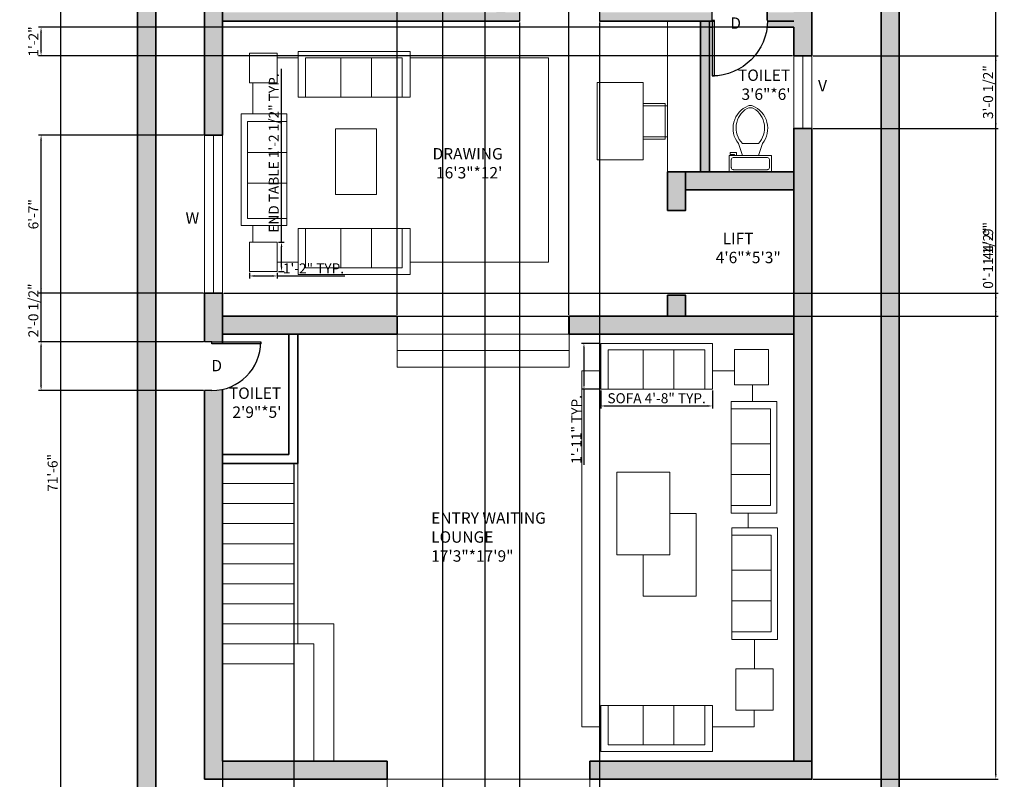
# Model space of a CAD drawing. Units: inches. Extents: x 2130 to 2621, y 981 to 1994.
# Tile 2 of 4: x 2130 to 2621, y 1353 to 1732. Entities that reach past the tile are written whole.
import ezdxf

# ---------------------------------------------------------------- set-up
doc = ezdxf.new("R2010")
doc.units = ezdxf.units.IN
for name, color, linetype, lineweight in [('A-ANNO-DIMS', 2, 'Continuous', 18), ('A-ANNO-TEXT', 10, 'Continuous', 18), ('A-AREA-IDEN', 10, 'Continuous', 18), ('A-FLOR-FIXT', 190, 'Continuous', 18), ('A-FLOR-STRS', 7, 'Continuous', 18), ('A-WALL-PATT', 140, 'Continuous', 13), ('C-PROP', 7, 'Continuous', 35), ('C-PROP-PATT', 140, 'Continuous', 13), ('DOOR', 130, 'Continuous', 25), ('FUR', 190, 'Continuous', 18), ('WALL', 140, 'Continuous', 35), ('WIND', 210, 'Continuous', 18)]:
    doc.layers.add(name, color=color, linetype=linetype, lineweight=lineweight)
doc.styles.get("Standard").update_dxf_attribs({"font": 'arial.ttf'})
doc.dimstyles.new('ISO-25', dxfattribs={"dimtxt": 5, "dimasz": 2.5, "dimexe": 1.25, "dimexo": 0.625, "dimtad": 1, "dimdec": 0, "dimlunit": 4, "dimtxsty": 'Standard', "dimcen": 2.5, "dimadec": 0, "dimazin": 0, "dimtfac": 1, "dimtdec": 0, "dimtmove": 0, "dimatfit": 3, "dimfxl": 1, "dimarcsym": 0})

# ---------------------------------------------------------------- blocks, each defined once
blk = doc.blocks.new('*U2')
for p, q in [((0, 0), (0, -6)), ((40, 0), (40, -6))]:
    blk.add_line(p, q)
blk.add_lwpolyline([(0, 0), (0, 40), (1.75, 40), (1.75, 0)], close=True)
blk.add_arc((0, 0), 40, 0, 90)
blk = doc.blocks.new('*D10')
at = {"layer": 'A-ANNO-DIMS', "color": 0, "lineweight": -2, "transparency": 16777216}
for p, q in [((2188.13, 1935.02), (2148.94, 1935.02)), ((2150.19, 1932.52), (2150.19, 1079.91)), ((2188.13, 1077.41), (2148.94, 1077.41))]:
    blk.add_line(p, q, dxfattribs=at)
at = {"layer": 'A-ANNO-DIMS', "color": 0, "transparency": 16777216}
for points in [[(2149.77, 1932.52), (2150.61, 1932.52), (2150.19, 1935.02)], [(2149.77, 1079.91), (2150.61, 1079.91), (2150.19, 1077.41)]]:
    blk.add_solid(points, dxfattribs=at)
at = {"layer": 'Defpoints', "color": 0, "transparency": 16777216}
for p in [(2188.76, 1935.02), (2150.19, 1077.41), (2188.76, 1077.41)]:
    blk.add_point(p, dxfattribs=at)
at = {"layer": 'A-ANNO-DIMS', "color": 0, "transparency": 16777216, "insert": (2147.01, 1506.21), "char_height": 5, "attachment_point": 5, "rotation": 90}
blk.add_mtext('71\'-6"', dxfattribs=at)
blk = doc.blocks.new('*U4')
for p, q in [((9.5, -6), (9.5, -2)), ((-10, -8.5), (-8, -8.5)), ((-10, -9.5), (-10, -8.5)), ((-7, -9.5), (-10, -9.5)), ((-8, -8.5), (-8, -8)), ((-7, -8), (-7, -9.5)), ((-4, -8), (-6, -14)), ((4, -8), (6, -14)), ((4, -14), (-4, -14))]:
    blk.add_line(p, q)
blk.add_lwpolyline([(10.5, -8), (10.5, 0), (-10.5, 0), (-10.5, -8)], close=True)
for points in [[(-9.5, -2), (-9.5, -6)], [(8.5, -1), (-8.5, -1)], [(-8.5, -7), (8.5, -7)]]:
    blk.add_lwpolyline(points)
for centre, radius, start, end in [((-8.62, -1.88), 0.884, 81.8699, 188.1301), ((8.62, -1.88), 0.884, 351.8699, 98.1301), ((-8.62, -6.12), 0.884, 171.8699, 278.1301), ((8.62, -6.12), 0.884, 261.8699, 8.1301), ((3.52, -21.58), 12.17, 141.4691, 247.9714), ((4.2, -21.82), 11.33, 136.3677, 238.9468), ((-3.52, -21.58), 12.17, 292.0284, 38.5307), ((-4.2, -21.82), 11.33, 301.053, 43.6321), ((0, -27.88), 4, 245.7318, 294.2682), ((0, -29), 4, 254.8605, 285.1395)]:
    blk.add_arc(centre, radius, start, end)
blk = doc.blocks.new('SOFA-THREE-SEAT')
for p, q in [((0, 0), (0, 55.76)), ((0, 55.76), (22.87, 55.76)), ((22.87, 55.76), (22.87, 51.91)), ((3.25, 36.47), (22.87, 36.47)), ((3.25, 21.24), (22.87, 21.24)), ((1.57, 0), (0, 0)), ((22.87, 0), (1.57, 0)), ((22.87, 3.65), (22.87, 0))]:
    blk.add_line(p, q)
blk.add_lwpolyline([(3.25, 3.65), (22.87, 3.65), (22.87, 51.91), (3.25, 51.91)], close=True)
blk = doc.blocks.new('TABLE-END')
blk.add_lwpolyline([(0, 14.67), (13.78, 14.67), (13.78, 0), (0, 0)], close=True)
blk = doc.blocks.new('*D15')
at = {"layer": 'A-ANNO-DIMS', "color": 0, "lineweight": -2, "transparency": 16777216}
for p, q in [((2419.82, 1547.31), (2419.82, 1538.32)), ((2475.58, 1547.31), (2475.58, 1538.32)), ((2422.32, 1539.57), (2473.08, 1539.57))]:
    blk.add_line(p, q, dxfattribs=at)
at = {"layer": 'A-ANNO-DIMS', "color": 0, "transparency": 16777216}
for points in [[(2422.32, 1539.99), (2422.32, 1539.16), (2419.82, 1539.57)], [(2473.08, 1539.99), (2473.08, 1539.16), (2475.58, 1539.57)]]:
    blk.add_solid(points, dxfattribs=at)
at = {"layer": 'Defpoints', "color": 0, "transparency": 16777216}
for p in [(2419.82, 1547.94), (2475.58, 1547.94), (2475.58, 1539.57)]:
    blk.add_point(p, dxfattribs=at)
at = {"layer": 'A-ANNO-DIMS', "color": 0, "transparency": 16777216, "insert": (2447.7, 1542.79), "char_height": 5, "attachment_point": 5}
blk.add_mtext('SOFA 4\'-8" TYP.', dxfattribs=at)
blk = doc.blocks.new('*D16')
at = {"layer": 'A-ANNO-DIMS', "color": 0, "lineweight": -2, "transparency": 16777216}
for p, q in [((2419.19, 1570.81), (2410.2, 1570.81)), ((2411.45, 1568.31), (2411.45, 1550.44)), ((2419.19, 1547.94), (2410.2, 1547.94)), ((2411.45, 1547.94), (2411.45, 1510.3))]:
    blk.add_line(p, q, dxfattribs=at)
at = {"layer": 'A-ANNO-DIMS', "color": 0, "transparency": 16777216}
for points in [[(2411.04, 1568.31), (2411.87, 1568.31), (2411.45, 1570.81)], [(2411.04, 1550.44), (2411.87, 1550.44), (2411.45, 1547.94)]]:
    blk.add_solid(points, dxfattribs=at)
at = {"layer": 'Defpoints', "color": 0, "transparency": 16777216}
for p in [(2419.82, 1570.81), (2411.45, 1547.94), (2419.82, 1547.94)]:
    blk.add_point(p, dxfattribs=at)
at = {"layer": 'A-ANNO-DIMS', "color": 0, "transparency": 16777216, "insert": (2408.32, 1527.87), "char_height": 5, "attachment_point": 5, "rotation": 90}
blk.add_mtext('1\'-11" TYP.', dxfattribs=at)
blk = doc.blocks.new('*D21')
at = {"layer": 'A-ANNO-DIMS', "color": 0, "lineweight": -2, "transparency": 16777216}
for p, q in [((2260.56, 1621.28), (2260.56, 1707.66)), ((2258.99, 1621.28), (2261.81, 1621.28)), ((2260.56, 1609.11), (2260.56, 1618.78)), ((2258.99, 1606.61), (2261.81, 1606.61))]:
    blk.add_line(p, q, dxfattribs=at)
at = {"layer": 'A-ANNO-DIMS', "color": 0, "transparency": 16777216}
for points in [[(2260.15, 1618.78), (2260.98, 1618.78), (2260.56, 1621.28)], [(2260.15, 1609.11), (2260.98, 1609.11), (2260.56, 1606.61)]]:
    blk.add_solid(points, dxfattribs=at)
at = {"layer": 'Defpoints', "color": 0, "transparency": 16777216}
for p in [(2258.36, 1621.28), (2260.56, 1621.28), (2258.36, 1606.61)]:
    blk.add_point(p, dxfattribs=at)
at = {"layer": 'A-ANNO-DIMS', "color": 0, "transparency": 16777216, "insert": (2257.35, 1665.72), "char_height": 5, "attachment_point": 5, "rotation": 90}
blk.add_mtext('END TABLE 1\'-2 1/2" TYP.', dxfattribs=at)
blk = doc.blocks.new('*D22')
at = {"layer": 'A-ANNO-DIMS', "color": 0, "lineweight": -2, "transparency": 16777216}
for p, q in [((2244.58, 1605.98), (2244.58, 1603.16)), ((2247.08, 1604.41), (2255.86, 1604.41)), ((2258.36, 1605.98), (2258.36, 1603.16)), ((2258.36, 1604.41), (2292.12, 1604.41))]:
    blk.add_line(p, q, dxfattribs=at)
at = {"layer": 'A-ANNO-DIMS', "color": 0, "transparency": 16777216}
for points in [[(2247.08, 1604.82), (2247.08, 1603.99), (2244.58, 1604.41)], [(2255.86, 1604.82), (2255.86, 1603.99), (2258.36, 1604.41)]]:
    blk.add_solid(points, dxfattribs=at)
at = {"layer": 'Defpoints', "color": 0, "transparency": 16777216}
for p in [(2244.58, 1606.61), (2258.36, 1606.61), (2258.36, 1604.41)]:
    blk.add_point(p, dxfattribs=at)
at = {"layer": 'A-ANNO-DIMS', "color": 0, "transparency": 16777216, "insert": (2276.49, 1607.54), "char_height": 5, "attachment_point": 5}
blk.add_mtext('1\'-2" TYP.', dxfattribs=at)
blk = doc.blocks.new('*D24')
at = {"layer": 'A-ANNO-DIMS', "color": 0, "lineweight": -2, "transparency": 16777216}
for p, q in [((2525.79, 1890.41), (2618.19, 1890.41)), ((2616.94, 1355.91), (2616.94, 1887.91)), ((2525.79, 1353.41), (2618.19, 1353.41))]:
    blk.add_line(p, q, dxfattribs=at)
at = {"layer": 'A-ANNO-DIMS', "color": 0, "transparency": 16777216}
for points in [[(2616.52, 1887.91), (2617.35, 1887.91), (2616.94, 1890.41)], [(2616.52, 1355.91), (2617.35, 1355.91), (2616.94, 1353.41)]]:
    blk.add_solid(points, dxfattribs=at)
at = {"layer": 'Defpoints', "color": 0, "transparency": 16777216}
for p in [(2525.16, 1890.41), (2616.94, 1890.41), (2525.16, 1353.41)]:
    blk.add_point(p, dxfattribs=at)
at = {"layer": 'A-ANNO-DIMS', "color": 0, "transparency": 16777216, "insert": (2613.76, 1621.91), "char_height": 5, "attachment_point": 5, "rotation": 90}
blk.add_mtext('44\'-9"', dxfattribs=at)
blk = doc.blocks.new('*D32')
at = {"layer": 'A-ANNO-DIMS', "color": 0, "lineweight": -2, "transparency": 16777216}
for p, q in [((2318.23, 1585.04), (2318.23, 1984.45)), ((2320.73, 1983.2), (2401.44, 1983.2)), ((2403.94, 1585.04), (2403.94, 1984.45))]:
    blk.add_line(p, q, dxfattribs=at)
at = {"layer": 'A-ANNO-DIMS', "color": 0, "transparency": 16777216}
for points in [[(2320.73, 1983.61), (2320.73, 1982.78), (2318.23, 1983.2)], [(2401.44, 1983.61), (2401.44, 1982.78), (2403.94, 1983.2)]]:
    blk.add_solid(points, dxfattribs=at)
at = {"layer": 'Defpoints', "color": 0, "transparency": 16777216}
for p in [(2403.94, 1983.2), (2318.23, 1584.41), (2403.94, 1584.41)]:
    blk.add_point(p, dxfattribs=at)
at = {"layer": 'A-ANNO-DIMS', "color": 0, "transparency": 16777216, "insert": (2361.08, 1986.41), "char_height": 5, "attachment_point": 5}
blk.add_mtext('7\'-1 1/2"', dxfattribs=at)
blk = doc.blocks.new('*D33')
at = {"layer": 'A-ANNO-DIMS', "color": 0, "lineweight": -2, "transparency": 16777216}
for p, q in [((2231.16, 1510.29), (2231.16, 984.42)), ((2266.66, 1510.29), (2266.66, 984.42)), ((2233.66, 985.67), (2264.16, 985.67))]:
    blk.add_line(p, q, dxfattribs=at)
at = {"layer": 'A-ANNO-DIMS', "color": 0, "transparency": 16777216}
for points in [[(2233.66, 986.08), (2233.66, 985.25), (2231.16, 985.67)], [(2264.16, 986.08), (2264.16, 985.25), (2266.66, 985.67)]]:
    blk.add_solid(points, dxfattribs=at)
at = {"layer": 'Defpoints', "color": 0, "transparency": 16777216}
for p in [(2231.16, 1510.91), (2266.66, 1510.91), (2266.66, 985.67)]:
    blk.add_point(p, dxfattribs=at)
at = {"layer": 'A-ANNO-DIMS', "color": 0, "transparency": 16777216, "insert": (2248.91, 988.88), "char_height": 5, "attachment_point": 5}
blk.add_mtext('2\'-11 1/2"', dxfattribs=at)
blk = doc.blocks.new('*D36')
at = {"layer": 'A-ANNO-DIMS', "color": 0, "lineweight": -2, "transparency": 16777216}
for p, q in [((2379.27, 1730.79), (2379.27, 984.42)), ((2419.27, 1730.79), (2419.27, 984.42)), ((2381.77, 985.67), (2416.77, 985.67))]:
    blk.add_line(p, q, dxfattribs=at)
at = {"layer": 'A-ANNO-DIMS', "color": 0, "transparency": 16777216}
for points in [[(2381.77, 986.08), (2381.77, 985.25), (2379.27, 985.67)], [(2416.77, 986.08), (2416.77, 985.25), (2419.27, 985.67)]]:
    blk.add_solid(points, dxfattribs=at)
at = {"layer": 'Defpoints', "color": 0, "transparency": 16777216}
for p in [(2379.27, 1731.41), (2419.27, 1731.41), (2419.27, 985.67)]:
    blk.add_point(p, dxfattribs=at)
at = {"layer": 'A-ANNO-DIMS', "color": 0, "transparency": 16777216, "insert": (2399.27, 988.85), "char_height": 5, "attachment_point": 5}
blk.add_mtext('3\'-4"', dxfattribs=at)
blk = doc.blocks.new('*D37')
at = {"layer": 'A-ANNO-DIMS', "color": 0, "lineweight": -2, "transparency": 16777216}
for p, q in [((2475.37, 1732.39), (2475.37, 1984.45)), ((2477.87, 1983.2), (2500.44, 1983.2)), ((2502.94, 1732.04), (2502.94, 1984.45))]:
    blk.add_line(p, q, dxfattribs=at)
at = {"layer": 'A-ANNO-DIMS', "color": 0, "transparency": 16777216}
for points in [[(2477.87, 1983.61), (2477.87, 1982.78), (2475.37, 1983.2)], [(2500.44, 1983.61), (2500.44, 1982.78), (2502.94, 1983.2)]]:
    blk.add_solid(points, dxfattribs=at)
at = {"layer": 'Defpoints', "color": 0, "transparency": 16777216}
for p in [(2502.94, 1983.2), (2475.37, 1731.77), (2502.94, 1731.41)]:
    blk.add_point(p, dxfattribs=at)
at = {"layer": 'A-ANNO-DIMS', "color": 0, "transparency": 16777216, "insert": (2489.15, 1986.41), "char_height": 5, "attachment_point": 5}
blk.add_mtext('2\'-3 1/2"', dxfattribs=at)
blk = doc.blocks.new('*D38')
at = {"layer": 'A-ANNO-DIMS', "color": 0, "lineweight": -2, "transparency": 16777216}
for p, q in [((2140.58, 1571.6), (2140.58, 1600.38)), ((2221.54, 1571.6), (2139.33, 1571.6)), ((2140.58, 1549.77), (2140.58, 1569.1)), ((2221.54, 1547.27), (2139.33, 1547.27))]:
    blk.add_line(p, q, dxfattribs=at)
at = {"layer": 'A-ANNO-DIMS', "color": 0, "transparency": 16777216}
for points in [[(2140.16, 1569.1), (2140.99, 1569.1), (2140.58, 1571.6)], [(2140.16, 1549.77), (2140.99, 1549.77), (2140.58, 1547.27)]]:
    blk.add_solid(points, dxfattribs=at)
at = {"layer": 'Defpoints', "color": 0, "transparency": 16777216}
for p in [(2140.58, 1571.6), (2222.16, 1571.6), (2222.16, 1547.27)]:
    blk.add_point(p, dxfattribs=at)
at = {"layer": 'A-ANNO-DIMS', "color": 0, "transparency": 16777216, "insert": (2137.37, 1587.24), "char_height": 5, "attachment_point": 5, "rotation": 90}
blk.add_mtext('2\'-0 1/2"', dxfattribs=at)
blk = doc.blocks.new('*D42')
at = {"layer": 'A-ANNO-DIMS', "color": 0, "lineweight": -2, "transparency": 16777216}
for p, q in [((2221.54, 1674.58), (2139.33, 1674.58)), ((2140.58, 1598.3), (2140.58, 1672.08)), ((2221.54, 1595.8), (2139.33, 1595.8))]:
    blk.add_line(p, q, dxfattribs=at)
at = {"layer": 'A-ANNO-DIMS', "color": 0, "transparency": 16777216}
for points in [[(2140.16, 1672.08), (2140.99, 1672.08), (2140.58, 1674.58)], [(2140.16, 1598.3), (2140.99, 1598.3), (2140.58, 1595.8)]]:
    blk.add_solid(points, dxfattribs=at)
at = {"layer": 'Defpoints', "color": 0, "transparency": 16777216}
for p in [(2140.58, 1674.58), (2222.16, 1674.58), (2222.16, 1595.8)]:
    blk.add_point(p, dxfattribs=at)
at = {"layer": 'A-ANNO-DIMS', "color": 0, "transparency": 16777216, "insert": (2137.4, 1635.19), "char_height": 5, "attachment_point": 5, "rotation": 90}
blk.add_mtext('6\'-7"', dxfattribs=at)
blk = doc.blocks.new('*D44')
at = {"layer": 'A-ANNO-DIMS', "color": 0, "lineweight": -2, "transparency": 16777216}
for p, q in [((2525.79, 1714.24), (2618.19, 1714.24)), ((2616.94, 1680.45), (2616.94, 1711.74)), ((2525.79, 1677.95), (2618.19, 1677.95))]:
    blk.add_line(p, q, dxfattribs=at)
at = {"layer": 'A-ANNO-DIMS', "color": 0, "transparency": 16777216}
for points in [[(2616.52, 1711.74), (2617.35, 1711.74), (2616.94, 1714.24)], [(2616.52, 1680.45), (2617.35, 1680.45), (2616.94, 1677.95)]]:
    blk.add_solid(points, dxfattribs=at)
at = {"layer": 'Defpoints', "color": 0, "transparency": 16777216}
for p in [(2525.16, 1714.24), (2616.94, 1714.24), (2525.16, 1677.95)]:
    blk.add_point(p, dxfattribs=at)
at = {"layer": 'A-ANNO-DIMS', "color": 0, "transparency": 16777216, "insert": (2613.72, 1696.09), "char_height": 5, "attachment_point": 5, "rotation": 90}
blk.add_mtext('3\'-0 1/2"', dxfattribs=at)
blk = doc.blocks.new('*D45')
at = {"layer": 'A-ANNO-DIMS', "color": 0, "lineweight": -2, "transparency": 16777216}
for p, q in [((2340.91, 1828.29), (2340.91, 984.42)), ((2361.98, 1828.29), (2361.98, 984.42)), ((2343.41, 985.67), (2359.48, 985.67))]:
    blk.add_line(p, q, dxfattribs=at)
at = {"layer": 'A-ANNO-DIMS', "color": 0, "transparency": 16777216}
for points in [[(2343.41, 986.08), (2343.41, 985.25), (2340.91, 985.67)], [(2359.48, 986.08), (2359.48, 985.25), (2361.98, 985.67)]]:
    blk.add_solid(points, dxfattribs=at)
at = {"layer": 'Defpoints', "color": 0, "transparency": 16777216}
for p in [(2340.91, 1828.91), (2361.98, 1828.91), (2361.98, 985.67)]:
    blk.add_point(p, dxfattribs=at)
at = {"layer": 'A-ANNO-DIMS', "color": 0, "transparency": 16777216, "insert": (2351.44, 988.84), "char_height": 5, "attachment_point": 5}
blk.add_mtext('1\'-9"', dxfattribs=at)
blk = doc.blocks.new('*D47')
at = {"layer": 'A-ANNO-DIMS', "color": 0, "lineweight": -2, "transparency": 16777216}
for p, q in [((2616.94, 1595.8), (2616.94, 1628.38)), ((2231.79, 1595.8), (2618.19, 1595.8)), ((2616.94, 1586.91), (2616.94, 1593.3)), ((2231.79, 1584.41), (2618.19, 1584.41))]:
    blk.add_line(p, q, dxfattribs=at)
at = {"layer": 'A-ANNO-DIMS', "color": 0, "transparency": 16777216}
for points in [[(2616.52, 1593.3), (2617.35, 1593.3), (2616.94, 1595.8)], [(2616.52, 1586.91), (2617.35, 1586.91), (2616.94, 1584.41)]]:
    blk.add_solid(points, dxfattribs=at)
at = {"layer": 'Defpoints', "color": 0, "transparency": 16777216}
for p in [(2231.16, 1595.8), (2616.94, 1595.8), (2231.16, 1584.41)]:
    blk.add_point(p, dxfattribs=at)
at = {"layer": 'A-ANNO-DIMS', "color": 0, "transparency": 16777216, "insert": (2613.73, 1613.34), "char_height": 5, "attachment_point": 5, "rotation": 90}
blk.add_mtext('0\'-11 1/2"', dxfattribs=at)
blk = doc.blocks.new('*D54')
at = {"layer": 'A-ANNO-DIMS', "color": 0, "lineweight": -2, "transparency": 16777216}
for p, q in [((2515.54, 1728.41), (2139.33, 1728.41)), ((2140.58, 1716.74), (2140.58, 1725.91)), ((2515.54, 1714.24), (2139.33, 1714.24))]:
    blk.add_line(p, q, dxfattribs=at)
at = {"layer": 'A-ANNO-DIMS', "color": 0, "transparency": 16777216}
for points in [[(2140.16, 1725.91), (2140.99, 1725.91), (2140.58, 1728.41)], [(2140.16, 1716.74), (2140.99, 1716.74), (2140.58, 1714.24)]]:
    blk.add_solid(points, dxfattribs=at)
at = {"layer": 'Defpoints', "color": 0, "transparency": 16777216}
for p in [(2140.58, 1728.41), (2516.16, 1728.41), (2516.16, 1714.24)]:
    blk.add_point(p, dxfattribs=at)
at = {"layer": 'A-ANNO-DIMS', "color": 0, "transparency": 16777216, "insert": (2137.44, 1721.33), "char_height": 5, "attachment_point": 5, "rotation": 90}
blk.add_mtext('1\'-2"', dxfattribs=at)

msp = doc.modelspace()

# ---------------------------------------------------------------- hatches: boundary and pattern name
at = {"layer": 'A-WALL-PATT'}
h = msp.add_hatch(color=256, dxfattribs=at)
h.dxf.hatch_style = 1
h.paths.add_polyline_path([(2272.17, 1886.91), (2272.17, 1890.41), (2222.16, 1890.41), (2222.16, 1870.49), (2231.16, 1870.49), (2231.16, 1881.41), (2272.82, 1881.41, -0.059514)])
h.paths.add_polyline_path([(2231.16, 1828.91), (2301.66, 1828.91), (2301.66, 1881.41), (2297.16, 1881.41), (2297.16, 1833.41), (2265.07, 1833.41), (2231.16, 1833.41), (2231.16, 1841.86), (2222.16, 1841.86), (2222.16, 1828.91), (2222.16, 1790.61), (2228.16, 1790.61, -0.01877), (2231.16, 1790.5)])
h.paths.add_polyline_path([(2303.95, 1886.91), (2303.95, 1890.41), (2301.66, 1890.41), (2295.51, 1890.41), (2295.51, 1886.91), (2295.51, 1881.41), (2297.16, 1881.41), (2301.66, 1881.41), (2303.95, 1881.41)])
h.paths.add_polyline_path([(2525.16, 1890.41), (2372.16, 1890.41), (2327.29, 1890.41), (2327.29, 1886.91, -0.059514), (2326.63, 1881.41), (2367.66, 1881.41), (2367.66, 1833.41), (2361.98, 1833.41), (2361.98, 1828.91), (2367.66, 1828.91), (2367.66, 1735.91), (2372.16, 1735.91), (2372.16, 1828.91), (2372.16, 1881.41), (2516.16, 1881.41), (2516.16, 1859.91), (2516.16, 1809.41), (2525.16, 1809.41)])
h.paths.add_polyline_path([(2475.37, 1735.91), (2419.27, 1735.91), (2419.27, 1731.41), (2475.37, 1731.41), (2475.37, 1731.77)])
h.paths.add_polyline_path([(2525.16, 1751.59), (2516.16, 1751.59), (2516.16, 1737.41), (2516.16, 1735.91), (2503, 1735.91), (2503, 1731.77, -0.030428), (2502.8, 1728.41), (2516.16, 1728.41), (2516.16, 1714.24), (2525.16, 1714.24), (2525.16, 1728.41)])
h.paths.add_polyline_path([(2379.27, 1735.91), (2231.16, 1735.91), (2231.16, 1731.41), (2379.27, 1731.41)])
h.paths.add_polyline_path([(2231.16, 1728.41), (2231.16, 1735.91), (2231.16, 1750.61), (2228.16, 1750.61), (2222.16, 1750.61), (2222.16, 1728.41), (2222.16, 1674.58), (2231.16, 1674.58)])
h.paths.add_polyline_path([(2516.16, 1584.41), (2462.16, 1584.41), (2403.94, 1584.41), (2403.94, 1575.41), (2404.07, 1575.41), (2453.16, 1575.41), (2516.16, 1575.41)], flags=17)
h.paths.add_polyline_path([(2516.16, 1584.41), (2462.16, 1584.41), (2403.94, 1584.41), (2403.94, 1575.41), (2453.16, 1575.41), (2516.16, 1575.41)], flags=17)
h.paths.add_polyline_path([(2318.23, 1584.41), (2231.16, 1584.41), (2231.16, 1575.41), (2318.23, 1575.41)])
h = msp.add_hatch(color=256, dxfattribs=at)
h.dxf.hatch_style = 1
h.paths.add_polyline_path([(2231.16, 1595.8), (2222.16, 1595.8), (2222.16, 1571.6), (2225.81, 1571.6), (2231.16, 1571.6)])
h.paths.add_polyline_path([(2313.28, 1362.41), (2237.26, 1362.41), (2231.16, 1362.41), (2231.16, 1404.41), (2231.16, 1474.85), (2231.16, 1547.86, -0.05547), (2225.81, 1547.27), (2222.16, 1547.27), (2222.16, 1425.41), (2222.16, 1353.41), (2313.28, 1353.41)])
h.paths.add_polyline_path([(2393.01, 1195.09), (2434.46, 1195.09), (2434.46, 1216.28), (2393.01, 1216.28)], flags=9)
h.paths.add_polyline_path([(2245.08, 1335), (2303.47, 1335), (2303.47, 1346.7), (2245.08, 1346.7)], flags=9)
h.paths.add_polyline_path([(2458.81, 1338.38), (2517.21, 1338.38), (2517.21, 1350.09), (2458.81, 1350.09)], flags=9)
h.paths.add_polyline_path([(2232.7, 1530.42), (2263.31, 1530.42), (2263.31, 1551.62), (2232.7, 1551.62)], flags=9)
h.paths.add_polyline_path([(2332.94, 1458.61), (2399.05, 1458.61), (2399.05, 1489.37), (2332.94, 1489.37)], flags=9)
h.paths.add_polyline_path([(2475.66, 1607.66), (2507.9, 1607.66), (2507.9, 1628.85), (2475.66, 1628.85)], flags=9)
h.paths.add_polyline_path([(2486.7, 1688.97), (2517.32, 1688.97), (2517.32, 1710.17), (2486.7, 1710.17)], flags=9)
h.paths.add_polyline_path([(2333.88, 1649.81), (2375.07, 1649.81), (2375.07, 1671), (2333.88, 1671)], flags=9)
h.paths.add_polyline_path([(2441.42, 1774.34), (2500.24, 1774.34), (2500.24, 1795.53), (2441.42, 1795.53)], flags=9)
h.paths.add_polyline_path([(2332.74, 1857.16), (2363.5, 1857.16), (2363.5, 1878.35), (2332.74, 1878.35)], flags=9)
h.paths.add_polyline_path([(2244.84, 1853.21), (2275.6, 1853.21), (2275.6, 1874.4), (2244.84, 1874.4)], flags=9)
h = msp.add_hatch(color=256, dxfattribs=at)
h.dxf.hatch_style = 1
h.paths.add_polyline_path([(2525.16, 1677.95), (2516.16, 1677.95), (2516.16, 1362.41), (2525.16, 1362.41)])
h.paths.add_polyline_path([(2516.16, 1656.41), (2462.16, 1656.41), (2462.16, 1647.41), (2516.16, 1647.41)])
h.paths.add_polyline_path([(2462.16, 1656.41), (2453.16, 1656.41), (2453.16, 1637.12), (2462.16, 1637.12)])
h.paths.add_polyline_path([(2474.15, 1731.41), (2469.66, 1731.41), (2469.66, 1656.41), (2474.15, 1656.41)])
h.paths.add_polyline_path([(2462.16, 1594.81), (2453.16, 1594.81), (2453.16, 1584.41), (2462.16, 1584.41)])
h.paths.add_polyline_path([(2516.16, 1584.41), (2404.07, 1584.41), (2404.07, 1575.41), (2516.16, 1575.41)])
h.paths.add_polyline_path([(2525.16, 1362.41), (2516.16, 1362.41), (2414.45, 1362.41), (2414.45, 1353.41), (2525.16, 1353.41)])
at = {"layer": 'C-PROP-PATT'}
h = msp.add_hatch(color=256, dxfattribs=at)
h.dxf.hatch_style = 1
h.paths.add_polyline_path([(2559.76, 1935.02), (2197.76, 1935.02), (2197.76, 1926.02), (2559.76, 1926.02)])
h.paths.add_polyline_path([(2197.76, 1935.02), (2188.76, 1935.02), (2188.76, 1077.41), (2197.76, 1077.41)])
h.paths.add_polyline_path([(2568.76, 1926.02), (2559.76, 1926.02), (2559.76, 1077.41), (2568.76, 1077.41)])
h.paths.add_polyline_path([(2568.76, 1935.02), (2559.76, 1935.02), (2559.76, 1926.02), (2568.76, 1926.02)])

# ---------------------------------------------------------------- linework, layer by layer
at = {"layer": 'A-FLOR-STRS'}
for p, q in [((2266.66, 1510.91), (2266.66, 1408.08)), ((2268.66, 1510.91), (2268.66, 1420.91)), ((2231.16, 1500.91), (2266.66, 1500.91)), ((2231.16, 1490.91), (2266.66, 1490.91)), ((2231.16, 1480.91), (2266.66, 1480.91)), ((2231.16, 1470.91), (2266.66, 1470.91)), ((2231.16, 1460.91), (2266.66, 1460.91)), ((2231.16, 1450.91), (2266.66, 1450.91)), ((2231.16, 1440.91), (2266.66, 1440.91)), ((2231.16, 1430.91), (2266.66, 1430.91)), ((2266.66, 1430.91), (2286.66, 1430.91)), ((2286.66, 1430.91), (2286.66, 1415.83)), ((2231.16, 1420.91), (2266.66, 1420.91)), ((2266.66, 1420.91), (2276.66, 1420.91)), ((2276.66, 1420.91), (2276.66, 1415.96)), ((2266.66, 1362.41), (2266.66, 1418.34)), ((2276.66, 1362.41), (2276.66, 1418.34)), ((2286.66, 1362.41), (2286.66, 1418.34)), ((2231.16, 1410.91), (2266.66, 1410.91)), ((2266.66, 1404.41), (2266.66, 1362.41))]:
    msp.add_line(p, q, dxfattribs=at)
for points in [[(2318.23, 1575.41), (2404.07, 1575.41), (2404.07, 1567.18), (2318.23, 1567.18)], [(2318.23, 1567.18), (2404.07, 1567.18), (2404.07, 1558.95), (2318.23, 1558.95)], [(2313.28, 1353.41), (2414.44, 1353.41), (2414.44, 1345.18), (2313.28, 1345.18)]]:
    msp.add_lwpolyline(points, close=True, dxfattribs=at)
at = {"layer": 'C-PROP'}
for p, q in [((2188.76, 1935.02), (2188.76, 1077.41)), ((2568.76, 1935.02), (2568.76, 1077.41)), ((2197.76, 1926.02), (2197.76, 1086.41)), ((2559.76, 1926.02), (2559.76, 1086.41))]:
    msp.add_line(p, q, dxfattribs=at)
for points in [[(2188.76, 1935.02), (2197.76, 1935.02), (2197.76, 1077.41), (2188.76, 1077.41)], [(2559.76, 1077.41), (2568.76, 1077.41), (2568.76, 1935.02), (2559.76, 1935.02)]]:
    msp.add_lwpolyline(points, close=True, dxfattribs=at)
at = {"layer": 'FUR'}
for p, q in [((2259.99, 1713.11), (2258.36, 1713.11)), ((2266.74, 1713.11), (2259.99, 1713.11)), ((2266.74, 1713.11), (2268.91, 1713.11)), ((2393.78, 1713.11), (2324.67, 1713.11)), ((2393.78, 1611.22), (2393.78, 1713.11)), ((2246.23, 1685.25), (2246.23, 1700.77)), ((2453.16, 1698.39), (2453.16, 1682.98)), ((2451.91, 1690.43), (2440.98, 1690.43)), ((2451.91, 1689.23), (2451.91, 1690.43)), ((2451.91, 1689.23), (2453.16, 1689.23)), ((2451.91, 1672.65), (2440.98, 1672.65)), ((2453.16, 1673.83), (2451.91, 1673.83)), ((2451.91, 1673.83), (2451.91, 1672.65)), ((2246.23, 1621.28), (2246.23, 1629.49)), ((2268.91, 1611.22), (2258.36, 1611.22)), ((2324.67, 1611.22), (2393.78, 1611.22)), ((2410.34, 1379.57), (2410.34, 1557.08)), ((2410.34, 1557.08), (2419.82, 1557.08)), ((2475.58, 1557.08), (2486.58, 1557.08)), ((2495.5, 1541.85), (2495.5, 1550.16)), ((2493.43, 1478.88), (2493.43, 1486.1)), ((2496.52, 1408.49), (2496.52, 1423.12)), ((2419.82, 1379.57), (2410.34, 1379.57))]:
    msp.add_line(p, q, dxfattribs=at)
for points in [[(2453.16, 1656.41), (2469.66, 1656.41), (2469.66, 1731.41), (2453.16, 1731.41)], [(2440.98, 1700.81), (2418.03, 1700.81), (2418.03, 1662.25), (2440.98, 1662.25)], [(2440.98, 1673.83), (2451.91, 1673.83), (2451.91, 1689.23), (2440.98, 1689.23)], [(2287.55, 1645.05), (2307.93, 1645.05), (2307.93, 1677.73), (2287.55, 1677.73)], [(2503.55, 1550.16), (2486.58, 1550.16), (2486.58, 1567.79), (2503.55, 1567.79)], [(2454.23, 1506.6), (2427.88, 1506.6), (2427.88, 1465.4), (2454.23, 1465.4)], [(2505.83, 1408.49), (2487.22, 1408.49), (2487.22, 1387.9), (2505.83, 1387.9)]]:
    msp.add_lwpolyline(points, close=True, dxfattribs=at)
for points in [[(2441.05, 1465.4), (2441.05, 1444.79), (2467.4, 1444.79), (2467.4, 1486), (2454.23, 1486)], [(2475.58, 1379.57), (2496.42, 1379.57), (2496.42, 1387.9)]]:
    msp.add_lwpolyline(points, dxfattribs=at)
at = {"layer": 'WALL'}
for p, q in [((2525.16, 1890.41), (2525.16, 1728.41)), ((2222.16, 1750.61), (2222.16, 1728.41)), ((2231.16, 1735.91), (2231.16, 1674.58)), ((2231.16, 1731.41), (2379.27, 1731.41)), ((2419.27, 1731.41), (2476.58, 1731.41)), ((2469.66, 1728.41), (2469.66, 1731.41)), ((2502.94, 1731.41), (2516.16, 1731.41)), ((2222.16, 1728.41), (2222.16, 1674.58)), ((2231.16, 1728.41), (2231.16, 1674.58)), ((2469.66, 1728.41), (2469.66, 1656.41)), ((2474.16, 1728.41), (2474.16, 1656.41)), ((2475.37, 1728.41), (2474.16, 1728.41)), ((2516.16, 1728.41), (2502.8, 1728.41)), ((2516.16, 1728.41), (2516.16, 1714.24)), ((2525.16, 1728.41), (2525.16, 1714.24)), ((2516.16, 1677.95), (2516.16, 1656.41)), ((2525.16, 1677.95), (2525.16, 1647.41)), ((2453.16, 1656.41), (2469.66, 1656.41)), ((2453.16, 1637.12), (2453.16, 1656.41)), ((2474.16, 1656.41), (2516.16, 1656.41)), ((2462.16, 1647.41), (2469.66, 1647.41)), ((2462.16, 1637.12), (2462.16, 1647.41)), ((2469.66, 1647.41), (2516.16, 1647.41)), ((2516.16, 1647.41), (2516.16, 1434.41)), ((2516.16, 1647.41), (2516.16, 1584.41)), ((2525.16, 1647.41), (2525.16, 1425.41)), ((2222.16, 1595.8), (2222.16, 1571.6)), ((2231.16, 1595.8), (2231.16, 1570.54)), ((2453.16, 1584.41), (2453.16, 1594.81)), ((2462.16, 1584.41), (2462.16, 1594.81)), ((2318.23, 1584.41), (2231.16, 1584.41)), ((2462.16, 1584.41), (2403.94, 1584.41)), ((2516.16, 1584.41), (2462.16, 1584.41)), ((2231.16, 1575.41), (2231.16, 1570.54)), ((2318.23, 1575.41), (2231.16, 1575.41)), ((2264.16, 1515.41), (2264.16, 1575.41)), ((2268.66, 1510.91), (2268.66, 1575.41)), ((2453.16, 1575.41), (2403.94, 1575.41)), ((2516.16, 1575.41), (2453.16, 1575.41)), ((2516.16, 1575.41), (2516.16, 1362.41)), ((2525.16, 1575.41), (2525.16, 1353.41)), ((2231.16, 1547.86), (2231.16, 1515.41)), ((2231.16, 1547.86), (2231.16, 1434.41)), ((2222.16, 1547.27), (2222.16, 1425.41)), ((2231.16, 1515.41), (2264.16, 1515.41)), ((2231.16, 1510.91), (2268.66, 1510.91)), ((2222.16, 1353.41), (2222.16, 1474.85)), ((2231.16, 1362.41), (2231.16, 1474.85)), ((2231.16, 1362.41), (2231.16, 1404.41)), ((2237.26, 1362.41), (2231.16, 1362.41)), ((2313.28, 1362.41), (2237.26, 1362.41)), ((2313.28, 1353.41), (2222.16, 1353.41))]:
    msp.add_line(p, q, dxfattribs=at)
for points in [[(2469.66, 1656.41), (2474.15, 1656.41), (2474.15, 1731.41), (2469.66, 1731.41)], [(2525.16, 1362.41), (2516.16, 1362.41), (2516.16, 1677.95), (2525.16, 1677.95)], [(2453.16, 1637.12), (2462.16, 1637.12), (2462.16, 1656.41), (2453.16, 1656.41)], [(2516.16, 1656.41), (2462.16, 1656.41), (2462.16, 1647.41), (2516.16, 1647.41)], [(2453.16, 1584.41), (2462.16, 1584.41), (2462.16, 1594.81), (2453.16, 1594.81)], [(2516.16, 1584.41), (2404.07, 1584.41), (2404.07, 1575.41), (2516.16, 1575.41)], [(2414.45, 1362.41), (2525.16, 1362.41), (2525.16, 1353.41), (2414.45, 1353.41)]]:
    msp.add_lwpolyline(points, close=True, dxfattribs=at)
for points in [[(2525.16, 1714.24), (2516.16, 1714.24)], [(2516.16, 1677.95), (2525.16, 1677.95)], [(2222.16, 1674.58), (2231.16, 1674.58)], [(2462.16, 1637.12), (2453.16, 1637.12)], [(2231.16, 1595.8), (2222.16, 1595.8)], [(2453.16, 1594.81), (2462.16, 1594.81)], [(2318.23, 1575.41), (2318.23, 1584.41)], [(2403.94, 1584.41), (2403.94, 1575.41)], [(2313.28, 1353.41), (2313.28, 1362.41)], [(2516.16, 1362.41), (2414.45, 1362.41), (2414.45, 1353.41), (2525.16, 1353.41)]]:
    msp.add_lwpolyline(points, dxfattribs=at)
at = {"layer": 'WIND'}
for p, q in [((2520.66, 1677.95), (2520.66, 1714.24)), ((2226.66, 1674.58), (2226.66, 1595.8))]:
    msp.add_line(p, q, dxfattribs=at)
for points in [[(2516.16, 1677.95), (2525.16, 1677.95), (2525.16, 1714.24), (2516.16, 1714.24)], [(2222.16, 1595.8), (2231.16, 1595.8), (2231.16, 1674.58), (2222.16, 1674.58)]]:
    msp.add_lwpolyline(points, close=True, dxfattribs=at)

# ---------------------------------------------------------------- block references
at = {"layer": 'A-FLOR-FIXT', "xscale": -1, "rotation": 180}
msp.add_blockref('*U4', (2494.48, 1656.41), dxfattribs=at)
at = {"layer": 'DOOR'}
msp.add_blockref('*U2', (2379.27, 1737.41), dxfattribs=at)
for p, xscale, yscale, zscale, rotation in [((2475.37, 1731.77), -0.6909314595712287, 0.6909314595712287, 0.6909314595712287, 180), ((2225.81, 1571.6), 0.6083677621983479, 0.6083677621983479, 0.6083677621983479, 270)]:
    msp.add_blockref('*U2', p, dxfattribs=dict(at, xscale=xscale, yscale=yscale, zscale=zscale, rotation=rotation))
at = {"layer": 'FUR'}
for name, p in [('TABLE-END', (2244.58, 1700.77)), ('SOFA-THREE-SEAT', (2240.39, 1629.49)), ('TABLE-END', (2244.58, 1606.61))]:
    msp.add_blockref(name, p, dxfattribs=at)
for p, rotation in [((2268.91, 1716.36), 270.0000000000012), ((2419.82, 1570.81), 270.0000000000003), ((2507.72, 1541.86), 180), ((2508.07, 1478.88), 180)]:
    msp.add_blockref('SOFA-THREE-SEAT', p, dxfattribs=dict(at, rotation=rotation))
at = {"layer": 'FUR', "extrusion": (0, 0, -1), "zscale": -1}
for p, rotation in [((-2268.91, 1605.14), 90.00000000000014), ((-2419.82, 1367.35), 89.99999999999923)]:
    msp.add_blockref('SOFA-THREE-SEAT', p, dxfattribs=dict(at, rotation=rotation))

# ---------------------------------------------------------------- texts
at = {"layer": 'A-ANNO-TEXT', "char_height": 5.68, "attachment_point": 1}
for s, insert in [('D', (2484.47, 1733.34)), ('V', (2528.25, 1702.08)), ('W', (2212.67, 1636.14)), ('D', (2225.54, 1562.53))]:
    msp.add_mtext_dynamic_manual_height_columns(s, width=39.9661, gutter_width=28.4, heights=[0], dxfattribs=dict(at, insert=insert))
at = {"layer": 'A-AREA-IDEN', "attachment_point": 1}
for s, width, insert, char_height in [('TOILET\\P 3\'6"*6\'', 39.9661, (2488.31, 1707.35), 5.68), ('DRAWING\\P 16\'3"*12\'', 39.9661, (2335.91, 1668.18), 5.68), ('  LIFT\\P4\'6"*5\'3"', 39.9661, (2477.18, 1625.93), 5.68), ('TOILET\\P 2\'9"*5\'', 39.9661, (2234.3, 1548.8), 5.68), ('ENTRY WAITING          \\PLOUNGE\\P17\'3"*17\'9"', 67.0335, (2335.22, 1486.54), 5.6797)]:
    msp.add_mtext_dynamic_manual_height_columns(s, width=width, gutter_width=28.4, heights=[0], dxfattribs=dict(at, insert=insert, char_height=char_height))

# ---------------------------------------------------------------- dimensions: what is measured, and where the dimension line sits
at = {"layer": 'A-ANNO-DIMS'}
for base, p1, p2, picture, middle in [((2403.94, 1983.2), (2318.23, 1584.41), (2403.94, 1584.41), '*D32', (2361.08, 1986.41)), ((2502.94, 1983.2), (2475.37, 1731.77), (2502.94, 1731.41), '*D37', (2489.15, 1986.41)), ((2361.98, 985.67), (2340.91, 1828.91), (2361.98, 1828.91), '*D45', (2351.44, 988.84)), ((2419.27, 985.67), (2379.27, 1731.41), (2419.27, 1731.41), '*D36', (2399.27, 988.85)), ((2266.66, 985.67), (2231.16, 1510.91), (2266.66, 1510.91), '*D33', (2248.91, 988.88))]:
    dim = msp.add_linear_dim(base=base, p1=p1, p2=p2, dimstyle='ISO-25', override={"dimdec": 1, "dimlfac": 1, "dimrnd": 0, "dimzin": 1, "dimdsep": 46, "dimlunit": 4, "dimfrac": 2}, dxfattribs=at)
    dim.commit()
    dim.dimension.update_dxf_attribs({"geometry": picture, "text_midpoint": middle})
for base, p1, p2, override, picture, middle in [((2150.19, 1077.41), (2188.76, 1935.02), (2188.76, 1077.41), {"dimclrd": 0, "dimclre": 0, "dimclrt": 0}, '*D10', (2147.01, 1506.21)), ((2616.94, 1890.41), (2525.16, 1353.41), (2525.16, 1890.41), {"dimdec": 1, "dimlfac": 1, "dimrnd": 0, "dimzin": 1, "dimdsep": 46, "dimlunit": 4, "dimfrac": 2}, '*D24', (2613.76, 1621.91)), ((2140.58, 1728.41), (2516.16, 1714.24), (2516.16, 1728.41), {"dimdec": 1, "dimlfac": 1, "dimrnd": 0, "dimzin": 1, "dimdsep": 46, "dimlunit": 4, "dimfrac": 2}, '*D54', (2137.44, 1721.33)), ((2616.94, 1714.24), (2525.16, 1677.95), (2525.16, 1714.24), {"dimdec": 1, "dimlfac": 1, "dimrnd": 0, "dimzin": 1, "dimdsep": 46, "dimlunit": 4, "dimfrac": 2}, '*D44', (2613.72, 1696.09)), ((2140.58, 1674.58), (2222.16, 1595.8), (2222.16, 1674.58), {"dimdec": 1, "dimlfac": 1, "dimrnd": 0, "dimzin": 1, "dimdsep": 46, "dimlunit": 4, "dimfrac": 2}, '*D42', (2137.4, 1635.19)), ((2616.94, 1595.8), (2231.16, 1584.41), (2231.16, 1595.8), {"dimdec": 1, "dimlfac": 1, "dimrnd": 0, "dimzin": 1, "dimdsep": 46, "dimlunit": 4, "dimfrac": 2}, '*D47', (2613.73, 1613.34)), ((2140.58, 1571.6), (2222.16, 1547.27), (2222.16, 1571.6), {"dimdec": 1, "dimlfac": 1, "dimrnd": 0, "dimzin": 1, "dimdsep": 46, "dimlunit": 4, "dimfrac": 2}, '*D38', (2137.37, 1587.24))]:
    dim = msp.add_linear_dim(base=base, p1=p1, p2=p2, angle=90, dimstyle='ISO-25', override=override, dxfattribs=at)
    dim.commit()
    dim.dimension.update_dxf_attribs({"geometry": picture, "text_midpoint": middle})
for base, p1, p2, angle, text, picture, middle in [((2260.56, 1621.28), (2258.36, 1606.61), (2258.36, 1621.28), 90, 'END TABLE <> TYP.', '*D21', (2257.35, 1665.72)), ((2411.45, 1547.94), (2419.82, 1570.81), (2419.82, 1547.94), 270, '<> TYP.', '*D16', (2408.32, 1527.87)), ((2475.58, 1539.57), (2419.82, 1547.94), (2475.58, 1547.94), 0, 'SOFA <> TYP.', '*D15', (2447.7, 1542.79))]:
    dim = msp.add_linear_dim(base=base, p1=p1, p2=p2, angle=angle, text=text, dimstyle='ISO-25', override={"dimdec": 1, "dimlfac": 1, "dimrnd": 0, "dimzin": 1, "dimdsep": 46, "dimlunit": 4, "dimfrac": 2}, dxfattribs=at)
    dim.commit()
    dim.dimension.update_dxf_attribs({"geometry": picture, "text_midpoint": middle})
dim = msp.add_linear_dim(base=(2258.36, 1604.41), p1=(2244.58, 1606.61), p2=(2258.36, 1606.61), text='<> TYP.', dimstyle='ISO-25', override={"dimdec": 1, "dimlfac": 1, "dimrnd": 0, "dimzin": 1, "dimdsep": 46, "dimlunit": 4, "dimfrac": 2}, dxfattribs=at)
dim.commit()
dim.dimension.update_dxf_attribs({"geometry": '*D22', "text_midpoint": (2276.49, 1607.54)})

doc.saveas('drawing.dxf')
